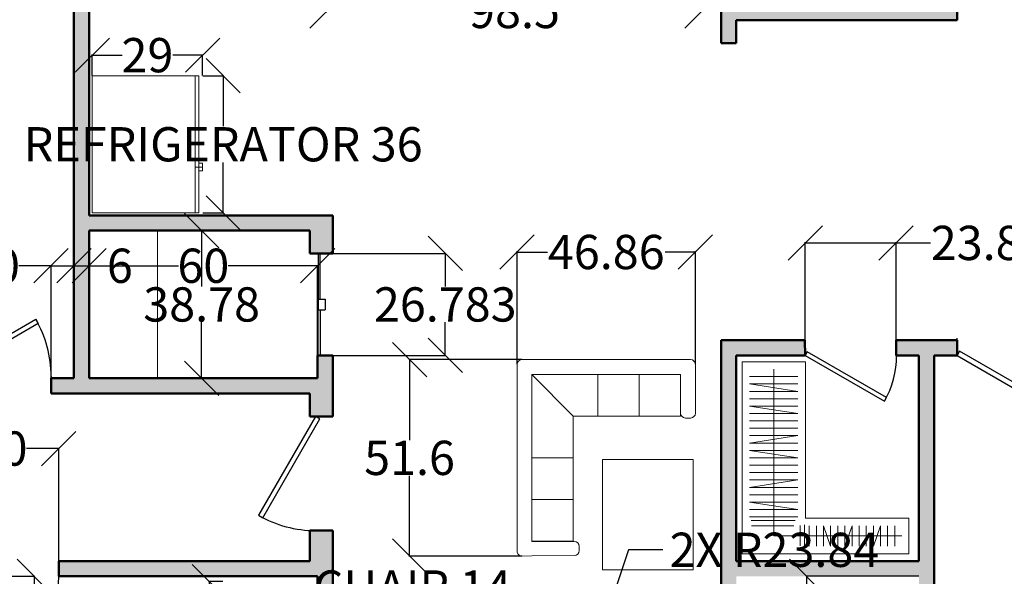
# Model space of a CAD drawing. Units: inches. Extents: x -9 to 615, y -420 to 89.
# Tile 3 of 6: x 201 to 460, y -261 to -115. Entities that reach past the tile are written whole.
import ezdxf

# ---------------------------------------------------------------- set-up
doc = ezdxf.new("R2010")
doc.units = ezdxf.units.IN
doc.header["$MEASUREMENT"] = 0
for name, color, linetype, lineweight in [('A-ANNO-DIMS', 2, 'Continuous', 18), ('A-DOOR', 4, 'Continuous', 25), ('A-EQPM', 8, 'Continuous', 18), ('A-FLOR-CASE', 32, 'Continuous', 18), ('A-FURN', 8, 'Continuous', 18), ('A-WALL', 7, 'Continuous', 50)]:
    doc.layers.add(name, color=color, linetype=linetype, lineweight=lineweight)
doc.layers.add('A-WALL-PATT', color=251, linetype='Continuous', lineweight=13, true_color=0x636466)
doc.styles.get("Standard").update_dxf_attribs({"font": 'arial.ttf'})
doc.dimstyles.get("Standard").update_dxf_attribs({"dimtxt": 9, "dimasz": 9, "dimexe": 0.18, "dimexo": 0.0625, "dimgap": 0.09, "dimtad": 0, "dimtih": 1, "dimtoh": 1, "dimdec": 0, "dimzin": 0, "dimdsep": 46, "dimlunit": 4, "dimtxsty": 'Standard', "dimblk": 'OBLIQUE', "dimblk2": 'OBLIQUE', "dimcen": 0.09, "dimadec": 0, "dimazin": 0, "dimtfac": 1, "dimtdec": 0, "dimtofl": 0, "dimtmove": 0, "dimatfit": 3, "dimldrblk": 'OBLIQUE', "dimfxl": 1, "dimtolj": 1, "dimtzin": 0, "dimarcsym": 0})

# ---------------------------------------------------------------- blocks, each defined once
blk = doc.blocks.new('Refrigerator-2 door - 36 in top')
for p, q in [((0, -26.999999), (36, -26.999999)), ((11, -27.999999), (11, -28.999999)), ((12, -26.999999), (12, -28.999999)), ((13, -28.999999), (13, -27.999999)), ((11, -28.999999), (13, -28.999999))]:
    blk.add_line(p, q)
blk.add_lwpolyline([(0, -27.999999), (0, 0), (36, 0), (36, -27.999999)], close=True)
blk = doc.blocks.new('*U14')
for p, q in [((0, 0), (0, 6)), ((40, 0), (40, 6))]:
    blk.add_line(p, q)
blk.add_lwpolyline([(0, 0), (40, 0), (40, 1.75), (0, 1.75)], close=True)
blk = doc.blocks.new('*U12')
for p, q in [((0, 0), (0, -6)), ((40, 0), (40, -6))]:
    blk.add_line(p, q)
blk.add_lwpolyline([(0, 0), (34.64, 20), (35.52, 18.48), (0.87, -1.52)], close=True)
blk.add_arc((0, 0), 40, 0, 30)
blk = doc.blocks.new('*U13')
for p, q in [((0, 0), (0, 6)), ((40, 0), (40, 6))]:
    blk.add_line(p, q)
blk.add_lwpolyline([(0, 0), (34.64, -20), (35.52, -18.48), (0.87, 1.52)], close=True)
blk.add_arc((0, 0), 40, 330, 0)
blk = doc.blocks.new('_Oblique')
at = {"color": 0, "linetype": 'ByBlock', "lineweight": -2}
blk.add_line((-0.5, -0.5), (0.5, 0.5), dxfattribs=at)
blk = doc.blocks.new('*D22')
at = {"layer": 'A-ANNO-DIMS', "color": 0, "lineweight": -2, "transparency": 16777216}
for p, q in [((254.55, -262.38), (250.83, -262.38)), ((251.01, -262.38), (251.01, -269.63)), ((251.01, -286.38), (251.01, -279.12)), ((254.55, -286.38), (250.83, -286.38))]:
    blk.add_line(p, q, dxfattribs=at)
at = {"layer": 'Defpoints', "color": 0, "transparency": 16777216}
for p in [(254.61, -262.38), (251.01, -286.38), (254.61, -286.38)]:
    blk.add_point(p, dxfattribs=at)
at = {"layer": 'A-ANNO-DIMS', "color": 0, "lineweight": -2, "transparency": 16777216, "xscale": 9, "yscale": 9, "zscale": 9}
for p, rotation in [((251.01, -262.38), 90), ((251.01, -286.38), 270)]:
    blk.add_blockref('_Oblique', p, dxfattribs=dict(at, rotation=rotation))
at = {"layer": 'A-ANNO-DIMS', "color": 0, "transparency": 16777216, "insert": (251.01, -274.38), "char_height": 9, "attachment_point": 5}
blk.add_mtext('\\A1;BASIN 24 TYP.', dxfattribs=at)
blk = doc.blocks.new('*D26')
at = {"layer": 'A-ANNO-DIMS', "color": 0, "lineweight": -2, "transparency": 16777216}
for p, q in [((281.97, -93.16), (281.97, -96.13)), ((300.94, -93.16), (300.94, -96.13)), ((281.97, -95.95), (300.94, -95.95)), ((300.94, -95.95), (309.94, -95.95))]:
    blk.add_line(p, q, dxfattribs=at)
at = {"layer": 'Defpoints', "color": 0, "transparency": 16777216}
for p in [(281.97, -93.1), (300.94, -93.1), (300.94, -95.95)]:
    blk.add_point(p, dxfattribs=at)
at = {"layer": 'A-ANNO-DIMS', "color": 0, "lineweight": -2, "transparency": 16777216, "xscale": 9, "yscale": 9, "zscale": 9, "rotation": 180}
blk.add_blockref('_Oblique', (281.97, -95.95), dxfattribs=at)
at = {"layer": 'A-ANNO-DIMS', "color": 0, "lineweight": -2, "transparency": 16777216, "xscale": 9, "yscale": 9, "zscale": 9}
blk.add_blockref('_Oblique', (300.94, -95.95), dxfattribs=at)
at = {"layer": 'A-ANNO-DIMS', "color": 0, "transparency": 16777216, "insert": (387.77, -95.95), "char_height": 9, "attachment_point": 5}
blk.add_mtext('\\A1;COUNTER STOOL 19 TYP.', dxfattribs=at)
blk = doc.blocks.new('*D28')
at = {"layer": 'A-ANNO-DIMS', "color": 0, "lineweight": -2, "transparency": 16777216}
for p, q in [((249.32, -129.53), (254.83, -129.53)), ((254.65, -129.53), (254.65, -142.78)), ((254.65, -165.53), (254.65, -152.28)), ((249.32, -165.53), (254.83, -165.53))]:
    blk.add_line(p, q, dxfattribs=at)
at = {"layer": 'Defpoints', "color": 0, "transparency": 16777216}
for p in [(249.25, -129.53), (254.65, -129.53), (249.25, -165.53)]:
    blk.add_point(p, dxfattribs=at)
at = {"layer": 'A-ANNO-DIMS', "color": 0, "lineweight": -2, "transparency": 16777216, "xscale": 9, "yscale": 9, "zscale": 9}
for p, rotation in [((254.65, -129.53), 90), ((254.65, -165.53), 270)]:
    blk.add_blockref('_Oblique', p, dxfattribs=dict(at, rotation=rotation))
at = {"layer": 'A-ANNO-DIMS', "color": 0, "transparency": 16777216, "insert": (254.65, -147.53), "char_height": 9, "attachment_point": 5}
blk.add_mtext('\\A1;REFRIGERATOR 36', dxfattribs=at)
blk = doc.blocks.new('*D29')
at = {"layer": 'A-ANNO-DIMS', "color": 0, "lineweight": -2, "transparency": 16777216}
for p, q in [((220.25, -129.47), (220.25, -123.95)), ((220.25, -124.13), (228.13, -124.13)), ((249.25, -124.13), (241.38, -124.13)), ((249.25, -129.47), (249.25, -123.95))]:
    blk.add_line(p, q, dxfattribs=at)
at = {"layer": 'Defpoints', "color": 0, "transparency": 16777216}
for p in [(220.25, -124.13), (220.25, -129.53), (249.25, -129.53)]:
    blk.add_point(p, dxfattribs=at)
at = {"layer": 'A-ANNO-DIMS', "color": 0, "lineweight": -2, "transparency": 16777216, "xscale": 9, "yscale": 9, "zscale": 9, "rotation": 180}
blk.add_blockref('_Oblique', (220.25, -124.13), dxfattribs=at)
at = {"layer": 'A-ANNO-DIMS', "color": 0, "lineweight": -2, "transparency": 16777216, "xscale": 9, "yscale": 9, "zscale": 9}
blk.add_blockref('_Oblique', (249.25, -124.13), dxfattribs=at)
at = {"layer": 'A-ANNO-DIMS', "color": 0, "transparency": 16777216, "insert": (234.75, -124.13), "char_height": 9, "attachment_point": 5}
blk.add_mtext('\\A1;29', dxfattribs=at)
blk = doc.blocks.new('*D30')
at = {"layer": 'A-ANNO-DIMS', "color": 0, "lineweight": -2, "transparency": 16777216}
for p, q in [((341.16, -263.93), (332.16, -263.93)), ((349.7, -266.78), (341.16, -263.93)), ((349.07, -268.67), (349.75, -266.61)), ((362.66, -271.11), (349.7, -266.78)), ((362.03, -272.99), (362.72, -270.94))]:
    blk.add_line(p, q, dxfattribs=at)
at = {"layer": 'Defpoints', "color": 0, "transparency": 16777216}
for p in [(349.05, -268.73), (349.7, -266.78), (362.01, -273.05)]:
    blk.add_point(p, dxfattribs=at)
at = {"layer": 'A-ANNO-DIMS', "color": 0, "lineweight": -2, "transparency": 16777216, "xscale": 9, "yscale": 9, "zscale": 9}
for p, rotation in [((349.7, -266.78), 161.5484668350482), ((362.66, -271.11), 341.5484668350483)]:
    blk.add_blockref('_Oblique', p, dxfattribs=dict(at, rotation=rotation))
at = {"layer": 'A-ANNO-DIMS', "color": 0, "transparency": 16777216, "insert": (304.39, -263.93), "char_height": 9, "attachment_point": 5}
blk.add_mtext('\\A1;CHAIR 14', dxfattribs=at)
blk = doc.blocks.new('*D42')
at = {"layer": 'A-ANNO-DIMS', "color": 0, "lineweight": -2, "transparency": 16777216}
for p, q in [((437.5, 54.02), (600.17, 54.02)), ((599.99, 54.02), (599.99, -160.45)), ((599.99, -384.29), (599.99, -169.82)), ((365.62, -384.29), (600.17, -384.29))]:
    blk.add_line(p, q, dxfattribs=at)
at = {"layer": 'Defpoints', "color": 0, "transparency": 16777216}
for p in [(437.44, 54.02), (599.99, 54.02), (365.56, -384.29)]:
    blk.add_point(p, dxfattribs=at)
at = {"layer": 'A-ANNO-DIMS', "color": 0, "lineweight": -2, "transparency": 16777216, "xscale": 9, "yscale": 9, "zscale": 9}
for p, rotation in [((599.99, 54.02), 90), ((599.99, -384.29), 270)]:
    blk.add_blockref('_Oblique', p, dxfattribs=dict(at, rotation=rotation))
at = {"layer": 'A-ANNO-DIMS', "color": 0, "transparency": 16777216, "insert": (599.99, -165.14), "char_height": 9, "attachment_point": 5}
blk.add_mtext('\\A1;438.3', dxfattribs=at)
blk = doc.blocks.new('*D62')
at = {"layer": 'A-ANNO-DIMS', "color": 0, "lineweight": -2, "transparency": 16777216}
for p, q in [((175.5, -260.98), (205.17, -260.98)), ((204.99, -260.98), (204.99, -292.37)), ((204.99, -332.98), (204.99, -301.59)), ((175.5, -332.98), (205.17, -332.98))]:
    blk.add_line(p, q, dxfattribs=at)
at = {"layer": 'Defpoints', "color": 0, "transparency": 16777216}
for p in [(175.44, -260.98), (175.44, -332.98), (204.99, -332.98)]:
    blk.add_point(p, dxfattribs=at)
at = {"layer": 'A-ANNO-DIMS', "color": 0, "lineweight": -2, "transparency": 16777216, "xscale": 9, "yscale": 9, "zscale": 9}
for p, rotation in [((204.99, -260.98), 90), ((204.99, -332.98), 270)]:
    blk.add_blockref('_Oblique', p, dxfattribs=dict(at, rotation=rotation))
at = {"layer": 'A-ANNO-DIMS', "color": 0, "transparency": 16777216, "insert": (204.99, -296.98), "char_height": 9, "attachment_point": 5}
blk.add_mtext('\\A1;72', dxfattribs=at)
blk = doc.blocks.new('*D63')
at = {"layer": 'A-ANNO-DIMS', "color": 0, "lineweight": -2, "transparency": 16777216}
for p, q in [((437.38, -260.98), (407.71, -260.98)), ((407.89, -260.98), (407.89, -292.37)), ((407.89, -332.98), (407.89, -301.59)), ((437.38, -332.98), (407.71, -332.98))]:
    blk.add_line(p, q, dxfattribs=at)
at = {"layer": 'Defpoints', "color": 0, "transparency": 16777216}
for p in [(407.89, -260.98), (437.44, -260.98), (437.44, -332.98)]:
    blk.add_point(p, dxfattribs=at)
at = {"layer": 'A-ANNO-DIMS', "color": 0, "lineweight": -2, "transparency": 16777216, "xscale": 9, "yscale": 9, "zscale": 9}
for p, rotation in [((407.89, -260.98), 90), ((407.89, -332.98), 270)]:
    blk.add_blockref('_Oblique', p, dxfattribs=dict(at, rotation=rotation))
at = {"layer": 'A-ANNO-DIMS', "color": 0, "transparency": 16777216, "insert": (407.89, -296.98), "char_height": 9, "attachment_point": 5}
blk.add_mtext('\\A1;72', dxfattribs=at)
blk = doc.blocks.new('*D67')
at = {"layer": 'A-ANNO-DIMS', "color": 0, "lineweight": -2, "transparency": 16777216}
for p, q in [((219.44, -208.92), (219.44, -179.25)), ((219.44, -179.43), (242.89, -179.43)), ((279.44, -179.43), (255.98, -179.43)), ((279.44, -208.92), (279.44, -179.25))]:
    blk.add_line(p, q, dxfattribs=at)
at = {"layer": 'Defpoints', "color": 0, "transparency": 16777216}
for p in [(279.44, -179.43), (219.44, -208.98), (279.44, -208.98)]:
    blk.add_point(p, dxfattribs=at)
at = {"layer": 'A-ANNO-DIMS', "color": 0, "lineweight": -2, "transparency": 16777216, "xscale": 9, "yscale": 9, "zscale": 9, "rotation": 180}
blk.add_blockref('_Oblique', (219.44, -179.43), dxfattribs=at)
at = {"layer": 'A-ANNO-DIMS', "color": 0, "lineweight": -2, "transparency": 16777216, "xscale": 9, "yscale": 9, "zscale": 9}
blk.add_blockref('_Oblique', (279.44, -179.43), dxfattribs=at)
at = {"layer": 'A-ANNO-DIMS', "color": 0, "transparency": 16777216, "insert": (249.44, -179.43), "char_height": 9, "attachment_point": 5}
blk.add_mtext('\\A1;60', dxfattribs=at)
blk = doc.blocks.new('*D68')
at = {"layer": 'A-ANNO-DIMS', "color": 0, "lineweight": -2, "transparency": 16777216}
for p, q in [((219.5, -170.2), (249.17, -170.2)), ((248.99, -170.2), (248.99, -184.9)), ((248.99, -208.98), (248.99, -194.28)), ((219.5, -208.98), (249.17, -208.98))]:
    blk.add_line(p, q, dxfattribs=at)
at = {"layer": 'Defpoints', "color": 0, "transparency": 16777216}
for p in [(219.44, -170.2), (219.44, -208.98), (248.99, -208.98)]:
    blk.add_point(p, dxfattribs=at)
at = {"layer": 'A-ANNO-DIMS', "color": 0, "lineweight": -2, "transparency": 16777216, "xscale": 9, "yscale": 9, "zscale": 9}
for p, rotation in [((248.99, -170.2), 90), ((248.99, -208.98), 270)]:
    blk.add_blockref('_Oblique', p, dxfattribs=dict(at, rotation=rotation))
at = {"layer": 'A-ANNO-DIMS', "color": 0, "transparency": 16777216, "insert": (248.99, -189.59), "char_height": 9, "attachment_point": 5}
blk.add_mtext('\\A1;38.78', dxfattribs=at)
blk = doc.blocks.new('*D69')
at = {"layer": 'A-ANNO-DIMS', "color": 0, "lineweight": -2, "transparency": 16777216}
for p, q in [((281.94, -83.03), (281.94, -112.7)), ((380.44, -83.03), (380.44, -112.7)), ((281.94, -112.52), (319.37, -112.52)), ((380.44, -112.52), (343, -112.52))]:
    blk.add_line(p, q, dxfattribs=at)
at = {"layer": 'Defpoints', "color": 0, "transparency": 16777216}
for p in [(281.94, -82.97), (380.44, -82.97), (281.94, -112.52)]:
    blk.add_point(p, dxfattribs=at)
at = {"layer": 'A-ANNO-DIMS', "color": 0, "lineweight": -2, "transparency": 16777216, "xscale": 9, "yscale": 9, "zscale": 9, "rotation": 180}
blk.add_blockref('_Oblique', (281.94, -112.52), dxfattribs=at)
at = {"layer": 'A-ANNO-DIMS', "color": 0, "lineweight": -2, "transparency": 16777216, "xscale": 9, "yscale": 9, "zscale": 9}
blk.add_blockref('_Oblique', (380.44, -112.52), dxfattribs=at)
at = {"layer": 'A-ANNO-DIMS', "color": 0, "transparency": 16777216, "insert": (331.19, -112.52), "char_height": 9, "attachment_point": 5}
blk.add_mtext('\\A1;98.5', dxfattribs=at)
blk = doc.blocks.new('*D77')
at = {"layer": 'A-ANNO-DIMS', "color": 0, "lineweight": -2, "transparency": 16777216}
for p, q in [((179.44, -208.92), (179.44, -179.25)), ((179.44, -179.43), (187.92, -179.43)), ((209.44, -179.43), (200.96, -179.43)), ((209.44, -208.92), (209.44, -179.25))]:
    blk.add_line(p, q, dxfattribs=at)
at = {"layer": 'Defpoints', "color": 0, "transparency": 16777216}
for p in [(209.44, -179.43), (179.44, -208.98), (209.44, -208.98)]:
    blk.add_point(p, dxfattribs=at)
at = {"layer": 'A-ANNO-DIMS', "color": 0, "lineweight": -2, "transparency": 16777216, "xscale": 9, "yscale": 9, "zscale": 9, "rotation": 180}
blk.add_blockref('_Oblique', (179.44, -179.43), dxfattribs=at)
at = {"layer": 'A-ANNO-DIMS', "color": 0, "lineweight": -2, "transparency": 16777216, "xscale": 9, "yscale": 9, "zscale": 9}
blk.add_blockref('_Oblique', (209.44, -179.43), dxfattribs=at)
at = {"layer": 'A-ANNO-DIMS', "color": 0, "transparency": 16777216, "insert": (194.44, -179.43), "char_height": 9, "attachment_point": 5}
blk.add_mtext('\\A1;30', dxfattribs=at)
blk = doc.blocks.new('*D78')
at = {"layer": 'A-ANNO-DIMS', "color": 0, "lineweight": -2, "transparency": 16777216}
for p, q in [((209.44, -208.92), (209.44, -179.25)), ((209.44, -179.43), (215.44, -179.43)), ((215.44, -208.92), (215.44, -179.25)), ((215.44, -179.43), (224.44, -179.43))]:
    blk.add_line(p, q, dxfattribs=at)
at = {"layer": 'Defpoints', "color": 0, "transparency": 16777216}
for p in [(215.44, -179.43), (209.44, -208.98), (215.44, -208.98)]:
    blk.add_point(p, dxfattribs=at)
at = {"layer": 'A-ANNO-DIMS', "color": 0, "lineweight": -2, "transparency": 16777216, "xscale": 9, "yscale": 9, "zscale": 9, "rotation": 180}
blk.add_blockref('_Oblique', (209.44, -179.43), dxfattribs=at)
at = {"layer": 'A-ANNO-DIMS', "color": 0, "lineweight": -2, "transparency": 16777216, "xscale": 9, "yscale": 9, "zscale": 9}
blk.add_blockref('_Oblique', (215.44, -179.43), dxfattribs=at)
at = {"layer": 'A-ANNO-DIMS', "color": 0, "transparency": 16777216, "insert": (227.5, -179.43), "char_height": 9, "attachment_point": 5}
blk.add_mtext('\\A1;6', dxfattribs=at)
blk = doc.blocks.new('*D80')
at = {"layer": 'A-ANNO-DIMS', "color": 0, "lineweight": -2, "transparency": 16777216}
for p, q in [((181.44, -256.92), (181.44, -227.25)), ((181.44, -227.43), (189.92, -227.43)), ((211.44, -227.43), (202.96, -227.43)), ((211.44, -256.92), (211.44, -227.25))]:
    blk.add_line(p, q, dxfattribs=at)
at = {"layer": 'Defpoints', "color": 0, "transparency": 16777216}
for p in [(211.44, -227.43), (181.44, -256.98), (211.44, -256.98)]:
    blk.add_point(p, dxfattribs=at)
at = {"layer": 'A-ANNO-DIMS', "color": 0, "lineweight": -2, "transparency": 16777216, "xscale": 9, "yscale": 9, "zscale": 9, "rotation": 180}
blk.add_blockref('_Oblique', (181.44, -227.43), dxfattribs=at)
at = {"layer": 'A-ANNO-DIMS', "color": 0, "lineweight": -2, "transparency": 16777216, "xscale": 9, "yscale": 9, "zscale": 9}
blk.add_blockref('_Oblique', (211.44, -227.43), dxfattribs=at)
at = {"layer": 'A-ANNO-DIMS', "color": 0, "transparency": 16777216, "insert": (196.44, -227.43), "char_height": 9, "attachment_point": 5}
blk.add_mtext('\\A1;30', dxfattribs=at)
blk = doc.blocks.new('*D83')
at = {"layer": 'A-ANNO-DIMS', "color": 0, "lineweight": -2, "transparency": 16777216}
for p, q in [((407.57, -202.92), (407.57, -173.25)), ((431.44, -202.92), (431.44, -173.25)), ((407.57, -173.43), (431.44, -173.43)), ((431.44, -173.43), (440.44, -173.43))]:
    blk.add_line(p, q, dxfattribs=at)
at = {"layer": 'Defpoints', "color": 0, "transparency": 16777216}
for p in [(431.44, -173.43), (407.57, -202.98), (431.44, -202.98)]:
    blk.add_point(p, dxfattribs=at)
at = {"layer": 'A-ANNO-DIMS', "color": 0, "lineweight": -2, "transparency": 16777216, "xscale": 9, "yscale": 9, "zscale": 9}
for p, rotation in [((407.57, -173.43), 179.9957313398861), ((431.44, -173.43), 359.995731339886)]:
    blk.add_blockref('_Oblique', p, dxfattribs=dict(at, rotation=rotation))
at = {"layer": 'A-ANNO-DIMS', "color": 0, "transparency": 16777216, "insert": (459.29, -173.43), "char_height": 9, "attachment_point": 5}
blk.add_mtext('\\A1;23.867', dxfattribs=at)
blk = doc.blocks.new('*D87')
at = {"layer": 'A-ANNO-DIMS', "color": 0, "lineweight": -2, "transparency": 16777216}
for p, q in [((331.86, -205.31), (331.86, -175.64)), ((331.86, -175.82), (339.84, -175.82)), ((378.72, -175.82), (370.74, -175.82)), ((378.72, -205.31), (378.72, -175.64))]:
    blk.add_line(p, q, dxfattribs=at)
at = {"layer": 'Defpoints', "color": 0, "transparency": 16777216}
for p in [(378.72, -175.82), (331.86, -205.37), (378.72, -205.37)]:
    blk.add_point(p, dxfattribs=at)
at = {"layer": 'A-ANNO-DIMS', "color": 0, "lineweight": -2, "transparency": 16777216, "xscale": 9, "yscale": 9, "zscale": 9, "rotation": 180}
blk.add_blockref('_Oblique', (331.86, -175.82), dxfattribs=at)
at = {"layer": 'A-ANNO-DIMS', "color": 0, "lineweight": -2, "transparency": 16777216, "xscale": 9, "yscale": 9, "zscale": 9}
blk.add_blockref('_Oblique', (378.72, -175.82), dxfattribs=at)
at = {"layer": 'A-ANNO-DIMS', "color": 0, "transparency": 16777216, "insert": (355.29, -175.82), "char_height": 9, "attachment_point": 5}
blk.add_mtext('\\A1;46.86', dxfattribs=at)
blk = doc.blocks.new('*D88')
at = {"layer": 'A-ANNO-DIMS', "color": 0, "lineweight": -2, "transparency": 16777216}
for p, q in [((333.1, -204.07), (303.43, -204.07)), ((303.61, -204.07), (303.61, -225.19)), ((303.62, -255.68), (303.62, -234.56)), ((333.11, -255.67), (303.44, -255.68))]:
    blk.add_line(p, q, dxfattribs=at)
at = {"layer": 'Defpoints', "color": 0, "transparency": 16777216}
for p in [(303.61, -204.07), (333.16, -204.07), (333.17, -255.67)]:
    blk.add_point(p, dxfattribs=at)
at = {"layer": 'A-ANNO-DIMS', "color": 0, "lineweight": -2, "transparency": 16777216, "xscale": 9, "yscale": 9, "zscale": 9}
for p, rotation in [((303.61, -204.07), 90.01273396399827), ((303.62, -255.68), 270.0127339639983)]:
    blk.add_blockref('_Oblique', p, dxfattribs=dict(at, rotation=rotation))
at = {"layer": 'A-ANNO-DIMS', "color": 0, "transparency": 16777216, "insert": (303.61, -229.88), "char_height": 9, "attachment_point": 5}
blk.add_mtext('\\A1;51.6', dxfattribs=at)
blk = doc.blocks.new('*D90')
at = {"layer": 'A-ANNO-DIMS', "color": 0, "lineweight": -2, "transparency": 16777216}
for p, q in [((283.5, -176.2), (313.17, -176.2)), ((312.99, -176.2), (312.99, -184.9)), ((312.99, -202.98), (312.99, -194.28)), ((283.5, -202.98), (313.17, -202.98))]:
    blk.add_line(p, q, dxfattribs=at)
at = {"layer": 'Defpoints', "color": 0, "transparency": 16777216}
for p in [(283.44, -176.2), (283.44, -202.98), (312.99, -202.98)]:
    blk.add_point(p, dxfattribs=at)
at = {"layer": 'A-ANNO-DIMS', "color": 0, "lineweight": -2, "transparency": 16777216, "xscale": 9, "yscale": 9, "zscale": 9}
for p, rotation in [((312.99, -176.2), 90), ((312.99, -202.98), 270)]:
    blk.add_blockref('_Oblique', p, dxfattribs=dict(at, rotation=rotation))
at = {"layer": 'A-ANNO-DIMS', "color": 0, "transparency": 16777216, "insert": (312.99, -189.59), "char_height": 9, "attachment_point": 5}
blk.add_mtext('\\A1;26.783', dxfattribs=at)
blk = doc.blocks.new('*D94')
at = {"layer": 'A-ANNO-DIMS', "color": 0, "lineweight": -2, "transparency": 16777216}
for p, q in [((361.16, -254.02), (355.46, -271.1)), ((370.16, -254.02), (361.16, -254.02)), ((347.83, -293.71), (348.01, -293.71)), ((347.92, -293.8), (347.92, -293.62))]:
    blk.add_line(p, q, dxfattribs=at)
at = {"layer": 'Defpoints', "color": 0, "transparency": 16777216}
for p in [(355.46, -271.1), (347.92, -293.71)]:
    blk.add_point(p, dxfattribs=at)
at = {"layer": 'A-ANNO-DIMS', "color": 0, "lineweight": -2, "transparency": 16777216, "xscale": 9, "yscale": 9, "zscale": 9, "rotation": 251.5488985370354}
blk.add_blockref('_Oblique', (355.46, -271.1), dxfattribs=at)
at = {"layer": 'A-ANNO-DIMS', "color": 0, "transparency": 16777216, "insert": (399.47, -254.02), "char_height": 9, "attachment_point": 5}
blk.add_mtext('\\A1;2X R23.84', dxfattribs=at)

msp = doc.modelspace()

# ---------------------------------------------------------------- hatches: boundary and pattern name
at = {"layer": 'A-WALL-PATT'}
h = msp.add_hatch(color=256, dxfattribs=at)
h.dxf.hatch_style = 1
h.paths.add_polyline_path([(389.4378, 18.0183), (30.4378, 18.0183), (30.4378, -341.9817), (316.4378, -341.9817), (316.4378, -336.5817), (316.4378, -332.9817), (283.4378, -332.9817), (283.4378, -256.9817), (283.4378, -250.9817), (283.4378, -248.9817), (278.9378, -248.9817), (277.4378, -248.9817), (277.4378, -250.9817), (277.4378, -256.9817), (211.4378, -256.9817), (211.4378, -260.9817), (279.4378, -260.9817), (279.4378, -332.9817), (175.4378, -332.9817), (175.4378, -260.9817), (181.4378, -260.9817), (181.4378, -256.9817), (175.4378, -256.9817), (175.4378, -248.9817), (171.4378, -248.9817), (171.4378, -332.9817), (39.4378, -332.9817), (39.4378, -212.9817), (171.4378, -212.9817), (171.4378, -218.9817), (175.4378, -218.9817), (175.4378, -212.9817), (179.4378, -212.9817), (179.4378, -208.9817), (135.4378, -208.9817), (135.4378, -114.9817), (179.4378, -114.9817), (179.4378, -110.9817), (100.4378, -110.9817), (100.4378, -114.9817), (131.4378, -114.9817), (131.4378, -208.9817), (39.4378, -208.9817), (39.4378, -114.9817), (70.4378, -114.9817), (70.4378, -110.9817), (39.4378, -110.9817), (39.4378, 9.0183), (215.4378, 9.0183), (215.4378, -110.9817), (215.4378, -208.9817), (209.4378, -208.9817), (209.4378, -212.9817), (215.4378, -212.9817), (255.4378, -212.9817), (277.4378, -212.9817), (277.4378, -218.9817), (283.4378, -218.9817), (283.4378, -212.9817), (283.4378, -208.9817), (283.4378, -202.9817), (279.4378, -202.9817), (279.4378, -208.9817), (255.4378, -208.9817), (219.4378, -208.9817), (219.4378, -170.1983), (255.4378, -170.1983), (277.4378, -170.1983), (277.4378, -176.1983), (283.4378, -176.1983), (283.4378, -170.1983), (283.4378, -166.1983), (255.4378, -166.1983), (219.4378, -166.1983), (219.4378, -42.9817), (243.4378, -42.9817), (243.4378, -38.9817), (219.4378, -38.9817), (219.4378, 9.0183), (267.4378, 9.0183), (267.4378, -38.9817), (261.4378, -38.9817), (261.4378, -42.9817), (271.4378, -42.9817), (271.4378, 9.0183), (380.4378, 9.0183), (380.4378, -14.9817), (380.4378, -23.9817), (401.4378, -23.9817), (401.4378, -14.9817), (389.4378, -14.9817)])
h = msp.add_hatch(color=256, dxfattribs=at)
h.dxf.hatch_style = 1
h.paths.add_polyline_path([(570.4378, 18.0183), (437.4378, 18.0183), (437.4378, -14.9817), (437.4378, -110.9817), (385.4378, -110.9817), (385.4378, -114.9817), (385.4378, -120.9817), (389.4378, -120.9817), (389.4378, -114.9817), (437.4378, -114.9817), (447.4378, -114.9817), (447.4378, -110.9817), (441.4378, -110.9817), (441.4378, 9.0183), (561.4378, 9.0183), (561.4378, -110.9817), (477.4378, -110.9817), (477.4378, -114.9817), (497.4378, -114.9817), (497.4378, -168.9817), (501.4378, -168.9817), (501.4378, -114.9817), (561.4378, -114.9817), (561.4378, -198.9817), (531.4378, -198.9817), (501.4378, -198.9817), (501.4378, -192.9817), (497.4378, -192.9817), (497.4378, -198.9817), (477.4378, -198.9817), (477.4378, -202.9817), (561.4378, -202.9817), (561.4378, -332.9817), (441.4378, -332.9817), (441.4378, -202.9817), (447.4378, -202.9817), (447.4378, -198.9817), (437.4378, -198.9817), (431.4378, -198.9817), (431.4378, -202.9817), (437.4378, -202.9817), (437.4378, -256.9817), (389.4378, -256.9817), (389.4378, -202.9799), (407.5704, -202.9799), (407.4511, -198.9817), (389.4378, -198.9817), (385.4378, -198.9817), (385.4378, -302.9817), (389.4378, -302.9817), (389.4378, -260.9817), (437.4378, -260.9817), (437.4378, -332.9817), (389.4378, -332.9817), (389.4378, -326.9817), (385.4378, -326.9817), (385.4378, -332.9817), (352.4378, -332.9817), (352.4378, -341.9817), (570.4378, -341.9817)])

# ---------------------------------------------------------------- linework, layer by layer
at = {"layer": 'A-DOOR'}
for p, q in [((279.6378, -188.1983), (279.6378, -190.9817)), ((281.4378, -188.1983), (281.4378, -190.9817))]:
    msp.add_line(p, q, dxfattribs=at)
at = {"layer": 'A-FLOR-CASE'}
for p, q in [((237.4378, -208.9817), (237.4378, -170.1983)), ((390.9651, -252.651), (390.9651, -204.651)), ((390.9651, -204.651), (407.6202, -204.651)), ((399.2926, -206.5905), (399.2926, -250.3886)), ((407.6202, -204.651), (407.6202, -245.7046)), ((392.9651, -208.5301), (405.6202, -208.5301)), ((392.9651, -210.4696), (405.6202, -210.4696)), ((392.9651, -210.4696), (405.6202, -212.4091)), ((392.9651, -212.4091), (405.6202, -212.4091)), ((392.9651, -214.3487), (405.6202, -214.3487)), ((392.9651, -216.2882), (405.6202, -216.2882)), ((392.9651, -216.2882), (405.6202, -218.2278)), ((392.9651, -218.2278), (405.6202, -218.2278)), ((392.9651, -220.1673), (405.6202, -220.1673)), ((392.9651, -222.1069), (405.6202, -222.1069)), ((392.9651, -224.0464), (405.6202, -224.0464)), ((405.6202, -224.0464), (392.9651, -225.986)), ((392.9651, -225.986), (405.6202, -225.986)), ((392.9651, -227.9255), (405.6202, -227.9255)), ((392.9651, -227.9255), (405.6202, -229.8651)), ((392.9651, -229.8651), (405.6202, -229.8651)), ((392.9651, -231.8046), (405.6202, -231.8046)), ((392.9651, -233.7442), (405.6202, -233.7442)), ((392.9651, -235.6837), (405.6202, -235.6837)), ((405.6202, -235.6837), (392.9651, -237.6233)), ((392.9651, -237.6233), (405.6202, -237.6233)), ((392.9651, -239.5628), (405.6202, -239.5628)), ((392.9651, -241.5023), (405.6202, -241.5023)), ((392.9651, -241.5023), (405.6202, -243.4419)), ((390.9651, -245.7046), (390.9651, -255.0727)), ((392.9651, -243.4419), (405.6202, -243.4419)), ((392.9651, -245.3814), (405.6202, -245.3814)), ((399.2926, -250.3886), (399.2926, -245.7046)), ((434.8024, -245.7046), (407.6202, -245.7046)), ((434.8024, -255.0727), (434.8024, -245.7046)), ((393.3348, -246.3322), (404.9567, -246.3322)), ((393.4756, -247.7391), (404.6045, -247.7391)), ((406.2245, -247.6688), (406.2245, -252.9447)), ((407.3515, -247.4577), (407.3515, -253.0854)), ((408.6373, -253.0727), (408.6373, -247.7046)), ((410.5062, -253.0727), (410.5062, -247.7046)), ((412.3752, -253.0727), (412.3752, -247.7046)), ((412.3752, -247.7046), (414.2441, -253.0727)), ((414.2441, -253.0727), (414.2441, -247.7046)), ((416.113, -253.0727), (416.113, -247.7046)), ((417.982, -253.0727), (417.982, -247.7046)), ((419.8509, -247.7046), (417.982, -253.0727)), ((419.8509, -253.0727), (419.8509, -247.7046)), ((421.7198, -253.0727), (421.7198, -247.7046)), ((423.5888, -253.0727), (423.5888, -247.7046)), ((425.4577, -253.0727), (425.4577, -247.7046)), ((427.3266, -247.7046), (425.4577, -253.0727)), ((427.3266, -253.0727), (427.3266, -247.7046)), ((429.1956, -253.0727), (429.1956, -247.7046)), ((431.0645, -253.0727), (431.0645, -247.7046)), ((432.9334, -250.3886), (399.2926, -250.3886)), ((390.9651, -255.0727), (434.8024, -255.0727))]:
    msp.add_line(p, q, dxfattribs=at)
at = {"layer": 'A-FURN'}
for p, q in [((377.4184, -204.0682), (333.1585, -204.0682)), ((331.8567, -205.37), (331.8567, -250.9316)), ((378.7201, -218.1187), (378.7201, -205.37)), ((335.762, -250.9316), (335.762, -207.9735)), ((335.762, -207.9735), (374.8148, -207.9735)), ((346.6233, -218.9199), (335.762, -207.9735)), ((374.8148, -207.9735), (374.8148, -218.1187)), ((376.1166, -219.4204), (377.4184, -219.4204)), ((331.8567, -250.9316), (331.8567, -254.3675)), ((335.762, -251.7411), (335.762, -251.8165)), ((346.8837, -251.8165), (335.762, -251.8165)), ((348.1953, -254.235), (348.1854, -253.1068)), ((335.762, -255.6464), (333.1699, -255.6692)), ((335.762, -255.6464), (346.9051, -255.5482))]:
    msp.add_line(p, q, dxfattribs=at)
for points in [[(346.6173, -218.9139), (353.0922, -218.9139), (353.0922, -207.9735), (342.2309, -207.9735)], [(335.762, -218.9199), (335.762, -229.8603), (346.6233, -229.8603), (346.6233, -218.9199)]]:
    msp.add_lwpolyline(points, dxfattribs=at)
for points in [[(363.9535, -207.9735), (353.0922, -207.9735), (353.0922, -218.9139), (363.9535, -218.9139)], [(374.8148, -207.9735), (363.9535, -207.9735), (363.9535, -218.9139), (374.8148, -218.9139)], [(346.6233, -229.8603), (335.762, -229.8603), (335.762, -240.8007), (346.6233, -240.8007)], [(354.3147, -230.3224), (378.1387, -230.3224), (378.1387, -259.3132), (354.3147, -259.3132)], [(346.6233, -240.8007), (335.762, -240.8007), (335.762, -251.7411), (346.6233, -251.7411)]]:
    msp.add_lwpolyline(points, close=True, dxfattribs=at)
for centre, start, end in [((333.1585, -205.37), 90, 180), ((377.4184, -205.37), 0, 90), ((376.1166, -218.1187), 180, 270), ((377.4184, -218.1187), 270, 0), ((346.8837, -253.1182), 0.504773, 90), ((333.1585, -254.3675), 180, 270.504773), ((346.8936, -254.2465), 270.504773, 0.504773)]:
    msp.add_arc(centre, 1.3018, start, end, dxfattribs=at)
at = {"layer": 'A-WALL'}
for p, q in [((215.4378, -208.9817), (215.4378, 9.0183)), ((219.4378, -166.1983), (219.4378, -42.9817)), ((385.4378, -110.9817), (385.4378, -114.9817)), ((447.4378, -110.9817), (447.4378, -114.9817)), ((385.4378, -120.9817), (385.4378, -114.9817)), ((385.4378, -114.9817), (385.4378, -120.9817)), ((389.4378, -114.9817), (437.4378, -114.9817)), ((389.4378, -120.9817), (389.4378, -114.9817)), ((437.4378, -114.9817), (447.4378, -114.9817)), ((385.4378, -120.9817), (389.4378, -120.9817)), ((255.4378, -166.1983), (219.4378, -166.1983)), ((283.4378, -166.1983), (255.4378, -166.1983)), ((283.4378, -170.1983), (283.4378, -166.1983)), ((219.4378, -208.9817), (219.4378, -170.1983)), ((219.4378, -170.1983), (255.4378, -170.1983)), ((255.4378, -170.1983), (277.4378, -170.1983)), ((277.4378, -176.1983), (277.4378, -170.1983)), ((283.4378, -170.1983), (283.4378, -176.1983)), ((283.4378, -176.1983), (277.4378, -176.1983)), ((385.4378, -198.9817), (385.4378, -302.9817)), ((385.4378, -198.9817), (389.4378, -198.9817)), ((389.4378, -198.9817), (407.4511, -198.9817)), ((407.4511, -198.9817), (407.5704, -202.9799)), ((437.4378, -198.9817), (431.4378, -198.9817)), ((431.4378, -198.9817), (431.4378, -202.9817)), ((437.4378, -198.9817), (447.4378, -198.9817)), ((447.4378, -202.9817), (447.4378, -198.9817)), ((283.4378, -202.9817), (279.4378, -202.9817)), ((279.4378, -202.9817), (279.4378, -208.9817)), ((283.4378, -208.9817), (283.4378, -202.9817)), ((389.4378, -202.9799), (389.4378, -256.9817)), ((407.5704, -202.9799), (389.4378, -202.9799)), ((431.4378, -202.9817), (437.4378, -202.9817)), ((437.4378, -202.9817), (437.4378, -256.9817)), ((441.4378, -202.9817), (447.4378, -202.9817)), ((441.4378, -202.9817), (441.4378, -332.9817)), ((215.4378, -208.9817), (209.4378, -208.9817)), ((209.4378, -208.9817), (209.4378, -212.9817)), ((255.4378, -208.9817), (219.4378, -208.9817)), ((279.4378, -208.9817), (255.4378, -208.9817)), ((283.4378, -212.9817), (283.4378, -208.9817)), ((215.4378, -212.9817), (209.4378, -212.9817)), ((215.4378, -212.9817), (255.4378, -212.9817)), ((255.4378, -212.9817), (277.4378, -212.9817)), ((277.4378, -218.9817), (277.4378, -212.9817)), ((283.4378, -212.9817), (283.4378, -218.9817)), ((283.4378, -218.9817), (277.4378, -218.9817)), ((277.4378, -250.9817), (277.4378, -248.9817)), ((277.4378, -248.9817), (283.4378, -248.9817)), ((283.4378, -248.9817), (283.4378, -250.9817)), ((277.4378, -250.9817), (277.4378, -256.9817)), ((283.4378, -256.9817), (283.4378, -250.9817)), ((277.4378, -256.9817), (211.4378, -256.9817)), ((211.4378, -256.9817), (211.4378, -260.9817)), ((283.4378, -332.9817), (283.4378, -256.9817)), ((437.4378, -256.9817), (389.4378, -256.9817)), ((279.4378, -260.9817), (211.4378, -260.9817)), ((279.4378, -332.9817), (279.4378, -260.9817))]:
    msp.add_line(p, q, dxfattribs=at)

# ---------------------------------------------------------------- block references
at = {"layer": 'A-DOOR'}
for name, p, xscale, yscale, zscale in [('*U12', (447.4378, -110.4817), 0.75, 0.75, 0.75), ('*U12', (179.4378, -208.4817), 0.75, 0.75, 0.75), ('*U13', (447.4378, -202.9817), 0.75, 0.75, 0.75), ('*U13', (407.5704, -202.9799), 0.6, 0.6, 0.6), ('*U13', (181.4378, -261.4817), 0.75, 0.75, 0.75)]:
    msp.add_blockref(name, p, dxfattribs=dict(at, xscale=xscale, yscale=yscale, zscale=zscale))
at = {"layer": 'A-DOOR', "rotation": 270}
for name, p, xscale, yscale, zscale in [('*U14', (279.6378, -176.1983), 0.3, 0.3, 0.3), ('*U14', (279.6378, -202.9817), -0.3, 0.3, 0.3), ('*U13', (278.9378, -218.9817), 0.75, 0.75, 0.75)]:
    msp.add_blockref(name, p, dxfattribs=dict(at, xscale=xscale, yscale=yscale, zscale=zscale))
at = {"layer": 'A-EQPM', "rotation": 90}
msp.add_blockref('Refrigerator-2 door - 36 in top', (220.2541, -165.5283), dxfattribs=at)

# ---------------------------------------------------------------- dimensions: what is measured, and where the dimension line sits
at = {"layer": 'A-ANNO-DIMS'}
for base, p1, p2, angle, override, picture, middle in [((599.9878, 54.0183), (365.5581, -384.2897), (437.4378, 54.0183), 90, {"dimdec": 1, "dimlfac": 1, "dimrnd": 0, "dimzin": 0, "dimdsep": 46, "dimlunit": 2}, '*D42', (599.9878, -165.1357)), ((281.9364, -112.5197), (380.4378, -82.9697), (281.9364, -82.9697), 180, {"dimdec": 1, "dimlfac": 1, "dimrnd": 0, "dimzin": 0, "dimdsep": 46, "dimlunit": 2}, '*D69', (331.1871, -112.5197)), ((220.2541, -124.1283), (249.2541, -129.5283), (220.2541, -129.5283), 180, {"dimdec": 0, "dimlfac": 1, "dimrnd": 0, "dimzin": 0, "dimdsep": 46, "dimlunit": 2}, '*D29', (234.7541, -124.1283)), ((248.9878, -208.9817), (219.4378, -170.1983), (219.4378, -208.9817), 270, {"dimdec": 2, "dimlfac": 1, "dimrnd": 0, "dimzin": 0, "dimdsep": 46, "dimlunit": 2}, '*D68', (248.9878, -189.59)), ((431.44, -173.4317), (407.5704, -202.9799), (431.4378, -202.9817), 359.995731, {"dimdec": 3, "dimlfac": 1, "dimrnd": 0, "dimzin": 0, "dimdsep": 46, "dimlunit": 2}, '*D83', (459.2882, -173.4324)), ((312.9878, -202.9817), (283.4378, -176.1983), (283.4378, -202.9817), 270, {"dimdec": 3, "dimlfac": 1, "dimrnd": 0, "dimzin": 0, "dimdsep": 46, "dimlunit": 2}, '*D90', (312.9878, -189.59)), ((303.6085, -204.0748), (333.1699, -255.6692), (333.1585, -204.0682), 90.012734, {"dimdec": 1, "dimlfac": 1, "dimrnd": 0, "dimzin": 0, "dimdsep": 46, "dimlunit": 2}, '*D88', (303.6142, -229.8753)), ((204.9878, -332.9817), (175.4378, -260.9817), (175.4378, -332.9817), 270, {"dimdec": 0, "dimlfac": 1, "dimrnd": 0, "dimzin": 0, "dimdsep": 46, "dimlunit": 2}, '*D62', (204.9878, -296.9817)), ((407.8878, -260.9817), (437.4378, -332.9817), (437.4378, -260.9817), 90, {"dimdec": 0, "dimlfac": 1, "dimrnd": 0, "dimzin": 0, "dimdsep": 46, "dimlunit": 2}, '*D63', (407.8878, -296.9817))]:
    dim = msp.add_linear_dim(base=base, p1=p1, p2=p2, angle=angle, dimstyle='Standard', override=override, dxfattribs=at)
    dim.commit()
    dim.dimension.update_dxf_attribs({"geometry": picture, "text_midpoint": middle})
dim = msp.add_linear_dim(base=(300.9428, -95.947), p1=(281.9733, -93.1016), p2=(300.9428, -93.1016), text='COUNTER STOOL <> TYP.', dimstyle='Standard', override={"dimdec": 0, "dimlfac": 1, "dimrnd": 0, "dimzin": 0, "dimdsep": 46, "dimlunit": 2}, dxfattribs=at)
dim.commit()
dim.dimension.update_dxf_attribs({"geometry": '*D26', "text_midpoint": (387.7699, -95.947)})
for base, p1, p2, angle, text, picture, middle in [((254.6541, -129.5283), (249.2541, -165.5283), (249.2541, -129.5283), 90, 'REFRIGERATOR <>', '*D28', (254.6541, -147.5283)), ((349.6979, -266.7831), (362.0148, -273.0541), (349.049, -268.728), 161.548467, 'CHAIR <>', '*D30', (304.3891, -263.9346)), ((251.0108, -286.3767), (254.6108, -262.3767), (254.6108, -286.3767), 270, 'BASIN <> TYP.', '*D22', (251.0108, -274.3767))]:
    dim = msp.add_linear_dim(base=base, p1=p1, p2=p2, angle=angle, text=text, dimstyle='Standard', override={"dimdec": 0, "dimlfac": 1, "dimrnd": 0, "dimzin": 0, "dimdsep": 46, "dimlunit": 2}, dxfattribs=at)
    dim.commit()
    dim.dimension.update_dxf_attribs({"geometry": picture, "text_midpoint": middle})
for base, p1, p2, override, picture, middle in [((378.7201, -175.82), (331.8567, -205.37), (378.7201, -205.37), {"dimdec": 2, "dimlfac": 1, "dimrnd": 0, "dimzin": 0, "dimdsep": 46, "dimlunit": 2}, '*D87', (355.2884, -175.82)), ((209.4378, -179.4317), (179.4378, -208.9817), (209.4378, -208.9817), {"dimdec": 0, "dimlfac": 1, "dimrnd": 0, "dimzin": 0, "dimdsep": 46, "dimlunit": 2}, '*D77', (194.4378, -179.4317)), ((215.4378, -179.4317), (209.4378, -208.9817), (215.4378, -208.9817), {"dimdec": 0, "dimlfac": 1, "dimrnd": 0, "dimzin": 0, "dimdsep": 46, "dimlunit": 2}, '*D78', (227.4991, -179.4317)), ((279.4378, -179.4317), (219.4378, -208.9817), (279.4378, -208.9817), {"dimdec": 0, "dimlfac": 1, "dimrnd": 0, "dimzin": 0, "dimdsep": 46, "dimlunit": 2}, '*D67', (249.4378, -179.4317)), ((211.4378, -227.4317), (181.4378, -256.9817), (211.4378, -256.9817), {"dimdec": 0, "dimlfac": 1, "dimrnd": 0, "dimzin": 0, "dimdsep": 46, "dimlunit": 2}, '*D80', (196.4378, -227.4317))]:
    dim = msp.add_linear_dim(base=base, p1=p1, p2=p2, dimstyle='Standard', override=override, dxfattribs=at)
    dim.commit()
    dim.dimension.update_dxf_attribs({"geometry": picture, "text_midpoint": middle})
dim = msp.add_radius_dim(center=(347.9183, -293.7099), mpoint=(355.4631, -271.0968), text='2X <>', dimstyle='Standard', override={"dimdec": 2, "dimlfac": 1, "dimrnd": 0, "dimzin": 0, "dimdsep": 46, "dimlunit": 2}, dxfattribs=at)
dim.commit()
dim.dimension.update_dxf_attribs({"geometry": '*D94', "text_midpoint": (399.4693, -254.0221)})

doc.saveas('drawing.dxf')
